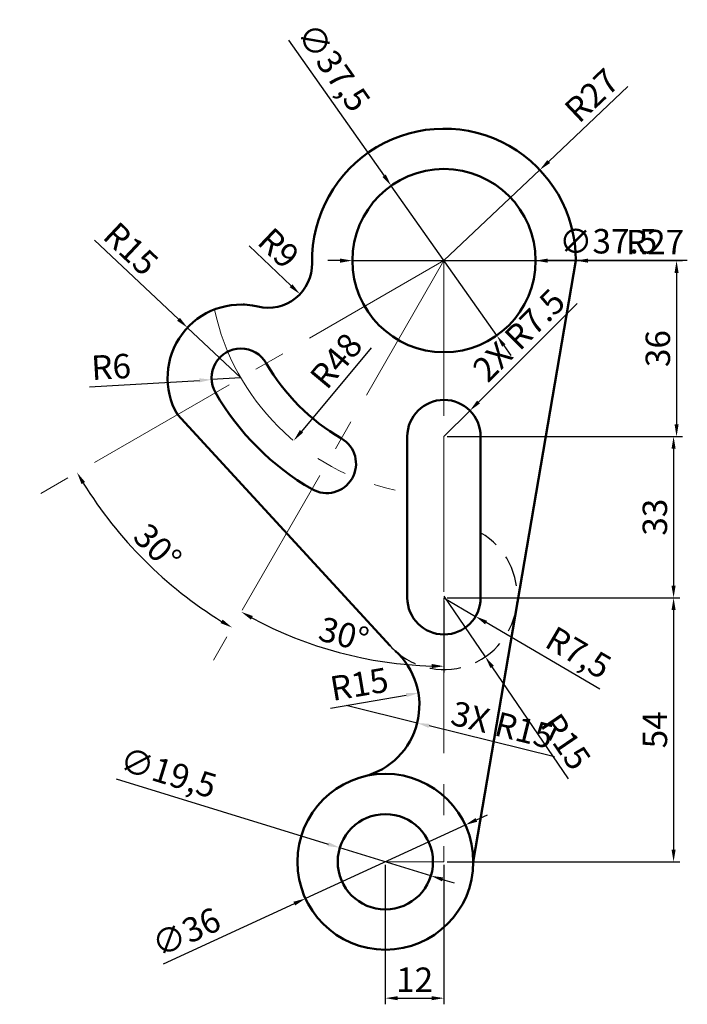
# Model space of a CAD drawing. Units: millimetres. Extents: x 3429 to 3566, y 1554 to 1755.
import ezdxf

# ---------------------------------------------------------------- set-up
doc = ezdxf.new("R2010")
doc.units = ezdxf.units.MM
doc.linetypes.add('CENTER', pattern=[50.8, 31.75, -6.35, 6.35, -6.35])
doc.linetypes.add('HIDDEN', pattern=[9.525, 6.35, -3.175])
for name, color, linetype, lineweight in [('M-CNTR', 4, 'CENTER', 18), ('M-DIMS', 2, 'Continuous', 25), ('M-HIDN', 7, 'HIDDEN', 25), ('M-OUTL', 7, 'Continuous', 50)]:
    doc.layers.add(name, color=color, linetype=linetype, lineweight=lineweight)
doc.styles.get("Standard").update_dxf_attribs({"font": 'arial.ttf'})
doc.dimstyles.new('ISO-25', dxfattribs={"dimtxt": 5, "dimasz": 2.5, "dimexe": 1.25, "dimexo": 0.625, "dimtad": 1, "dimtxsty": 'Standard', "dimcen": 2.5, "dimadec": 0, "dimazin": 0, "dimtfac": 1, "dimtmove": 0, "dimatfit": 3, "dimfxl": 1, "dimarcsym": 0})

# ---------------------------------------------------------------- blocks, each defined once
blk = doc.blocks.new('*D1')
at = {"layer": 'Defpoints', "color": 0, "transparency": 16777216}
for p in [(3516.16, 1705.91), (3516.16, 1669.91), (3563.76, 1669.91)]:
    blk.add_point(p, dxfattribs=at)
at = {"layer": 'M-DIMS', "color": 0, "lineweight": -2, "transparency": 16777216}
for p, q in [((3516.79, 1705.91), (3565.01, 1705.91)), ((3563.76, 1703.41), (3563.76, 1672.41)), ((3516.79, 1669.91), (3565.01, 1669.91))]:
    blk.add_line(p, q, dxfattribs=at)
at = {"layer": 'M-DIMS', "color": 0, "transparency": 16777216}
for points in [[(3563.35, 1703.41), (3564.18, 1703.41), (3563.76, 1705.91)], [(3563.35, 1672.41), (3564.18, 1672.41), (3563.76, 1669.91)]]:
    blk.add_solid(points, dxfattribs=at)
at = {"layer": 'M-DIMS', "color": 0, "transparency": 16777216, "insert": (3560.58, 1687.91), "char_height": 5, "attachment_point": 5, "rotation": 90}
blk.add_mtext('36', dxfattribs=at)
blk = doc.blocks.new('*D2')
at = {"layer": 'Defpoints', "color": 0, "transparency": 16777216}
for p in [(3516.16, 1669.91), (3516.16, 1636.91), (3563.15, 1636.91)]:
    blk.add_point(p, dxfattribs=at)
at = {"layer": 'M-DIMS', "color": 0, "lineweight": -2, "transparency": 16777216}
for p, q in [((3516.79, 1669.91), (3564.4, 1669.91)), ((3563.15, 1667.41), (3563.15, 1639.41)), ((3516.79, 1636.91), (3564.4, 1636.91))]:
    blk.add_line(p, q, dxfattribs=at)
at = {"layer": 'M-DIMS', "color": 0, "transparency": 16777216}
for points in [[(3562.73, 1667.41), (3563.57, 1667.41), (3563.15, 1669.91)], [(3562.73, 1639.41), (3563.57, 1639.41), (3563.15, 1636.91)]]:
    blk.add_solid(points, dxfattribs=at)
at = {"layer": 'M-DIMS', "color": 0, "transparency": 16777216, "insert": (3559.97, 1653.41), "char_height": 5, "attachment_point": 5, "rotation": 90}
blk.add_mtext('33', dxfattribs=at)
blk = doc.blocks.new('*D3')
at = {"layer": 'Defpoints', "color": 0, "transparency": 16777216}
for p in [(3516.16, 1636.91), (3516.16, 1582.91), (3563.15, 1582.91)]:
    blk.add_point(p, dxfattribs=at)
at = {"layer": 'M-DIMS', "color": 0, "lineweight": -2, "transparency": 16777216}
for p, q in [((3516.79, 1636.91), (3564.4, 1636.91)), ((3563.15, 1634.41), (3563.15, 1585.41)), ((3516.79, 1582.91), (3564.4, 1582.91))]:
    blk.add_line(p, q, dxfattribs=at)
at = {"layer": 'M-DIMS', "color": 0, "transparency": 16777216}
for points in [[(3562.73, 1634.41), (3563.57, 1634.41), (3563.15, 1636.91)], [(3562.73, 1585.41), (3563.57, 1585.41), (3563.15, 1582.91)]]:
    blk.add_solid(points, dxfattribs=at)
at = {"layer": 'M-DIMS', "color": 0, "transparency": 16777216, "insert": (3559.98, 1609.91), "char_height": 5, "attachment_point": 5, "rotation": 90}
blk.add_mtext('54', dxfattribs=at)
blk = doc.blocks.new('*D4')
at = {"layer": 'Defpoints', "color": 0, "transparency": 16777216}
for p in [(3504.16, 1582.91), (3516.16, 1582.91), (3516.16, 1555)]:
    blk.add_point(p, dxfattribs=at)
at = {"layer": 'M-DIMS', "color": 0, "lineweight": -2, "transparency": 16777216}
for p, q in [((3504.16, 1582.29), (3504.16, 1553.75)), ((3516.16, 1582.29), (3516.16, 1553.75)), ((3506.66, 1555), (3513.66, 1555))]:
    blk.add_line(p, q, dxfattribs=at)
at = {"layer": 'M-DIMS', "color": 0, "transparency": 16777216}
for points in [[(3506.66, 1555.41), (3506.66, 1554.58), (3504.16, 1555)], [(3513.66, 1555.41), (3513.66, 1554.58), (3516.16, 1555)]]:
    blk.add_solid(points, dxfattribs=at)
at = {"layer": 'M-DIMS', "color": 0, "transparency": 16777216, "insert": (3510.16, 1558.13), "char_height": 5, "attachment_point": 5}
blk.add_mtext('12', dxfattribs=at)
blk = doc.blocks.new('*D5')
at = {"layer": 'Defpoints', "color": 0, "transparency": 16777216}
for p in [(3516.16, 1705.91), (3516.16, 1669.91), (3516.16, 1636.91), (3487.78, 1627.93), (3468.96, 1624.15)]:
    blk.add_point(p, dxfattribs=at)
at = {"layer": 'M-DIMS', "color": 0, "lineweight": -2, "transparency": 16777216}
blk.add_line((3516.16, 1636.29), (3516.16, 1621.67), dxfattribs=at)
blk.add_arc((3516.16, 1705.91), 82.99, 241.7261, 268.2739, dxfattribs=at)
at = {"layer": 'M-DIMS', "color": 0, "transparency": 16777216}
for points in [[(3476.65, 1632.46), (3477.06, 1633.19), (3474.67, 1634.04)], [(3513.67, 1623.38), (3513.66, 1622.54), (3516.16, 1622.92)]]:
    blk.add_solid(points, dxfattribs=at)
at = {"layer": 'M-DIMS', "color": 0, "transparency": 16777216, "insert": (3495.51, 1628.82), "char_height": 5, "attachment_point": 5, "rotation": 345}
blk.add_mtext('30°', dxfattribs=at)
blk = doc.blocks.new('*D6')
at = {"layer": 'Defpoints', "color": 0, "transparency": 16777216}
for p in [(3535.78, 1724.47), (3516.16, 1705.91)]:
    blk.add_point(p, dxfattribs=at)
at = {"layer": 'M-DIMS', "color": 0, "lineweight": -2, "transparency": 16777216}
for p, q in [((3553.79, 1741.51), (3537.59, 1726.18)), ((3516.16, 1705.91), (3535.78, 1724.47))]:
    blk.add_line(p, q, dxfattribs=at)
at = {"layer": 'M-DIMS', "color": 0, "transparency": 16777216}
blk.add_solid([(3537.31, 1726.49), (3537.88, 1725.88), (3535.78, 1724.47)], dxfattribs=at)
at = {"layer": 'M-DIMS', "color": 0, "transparency": 16777216, "insert": (3546.85, 1739.25), "char_height": 5, "attachment_point": 5, "rotation": 43.4094}
blk.add_mtext('R27', dxfattribs=at)
blk = doc.blocks.new('*D7')
at = {"layer": 'Defpoints', "color": 0, "transparency": 16777216}
for p in [(3510.92, 1617.43), (3496.13, 1614.92)]:
    blk.add_point(p, dxfattribs=at)
at = {"layer": 'M-DIMS', "color": 0, "lineweight": -2, "transparency": 16777216}
blk.add_line((3492.94, 1614.37), (3508.45, 1617.01), dxfattribs=at)
at = {"layer": 'M-DIMS', "color": 0, "transparency": 16777216}
blk.add_solid([(3508.38, 1617.42), (3508.52, 1616.6), (3510.92, 1617.43)], dxfattribs=at)
at = {"layer": 'M-DIMS', "color": 0, "transparency": 16777216, "insert": (3498.93, 1618.62), "char_height": 5, "attachment_point": 5, "rotation": 9.6568}
blk.add_mtext('R15', dxfattribs=at)
blk = doc.blocks.new('*D8')
at = {"layer": 'Defpoints', "color": 0, "transparency": 16777216}
for p in [(3516.16, 1636.91), (3522.63, 1633.12)]:
    blk.add_point(p, dxfattribs=at)
at = {"layer": 'M-DIMS', "color": 0, "lineweight": -2, "transparency": 16777216}
for p, q in [((3516.16, 1636.91), (3522.63, 1633.12)), ((3548.08, 1618.2), (3524.79, 1631.85))]:
    blk.add_line(p, q, dxfattribs=at)
at = {"layer": 'M-DIMS', "color": 0, "transparency": 16777216}
blk.add_solid([(3525, 1632.21), (3524.58, 1631.49), (3522.63, 1633.12)], dxfattribs=at)
at = {"layer": 'M-DIMS', "color": 0, "transparency": 16777216, "insert": (3543.37, 1625.16), "char_height": 5, "attachment_point": 5, "rotation": 329.6153}
blk.add_mtext('R7,5', dxfattribs=at)
blk = doc.blocks.new('*D9')
at = {"layer": 'Defpoints', "color": 0, "transparency": 16777216}
for p in [(3516.16, 1637.25), (3524.61, 1624.85)]:
    blk.add_point(p, dxfattribs=at)
at = {"layer": 'M-DIMS', "color": 0, "lineweight": -2, "transparency": 16777216}
for p, q in [((3516.16, 1637.25), (3524.61, 1624.85)), ((3541.66, 1599.85), (3526.02, 1622.79))]:
    blk.add_line(p, q, dxfattribs=at)
at = {"layer": 'M-DIMS', "color": 0, "transparency": 16777216}
blk.add_solid([(3526.37, 1623.02), (3525.68, 1622.55), (3524.61, 1624.85)], dxfattribs=at)
at = {"layer": 'M-DIMS', "color": 0, "transparency": 16777216, "insert": (3540.56, 1607.11), "char_height": 5, "attachment_point": 5, "rotation": 304.2901}
blk.add_mtext('R15', dxfattribs=at)
blk = doc.blocks.new('*D10')
at = {"layer": 'Defpoints', "color": 0, "transparency": 16777216}
for p in [(3516.16, 1705.91), (3485.4, 1669.06)]:
    blk.add_point(p, dxfattribs=at)
at = {"layer": 'M-DIMS', "color": 0, "lineweight": -2, "transparency": 16777216}
blk.add_line((3501.25, 1688.04), (3487, 1670.98), dxfattribs=at)
at = {"layer": 'M-DIMS', "color": 0, "transparency": 16777216}
blk.add_solid([(3486.68, 1671.25), (3487.32, 1670.72), (3485.4, 1669.06)], dxfattribs=at)
at = {"layer": 'M-DIMS', "color": 0, "transparency": 16777216, "insert": (3494.58, 1685.01), "char_height": 5, "attachment_point": 5, "rotation": 50.1415}
blk.add_mtext('R48', dxfattribs=at)
blk = doc.blocks.new('*D11')
at = {"layer": 'Defpoints', "color": 0, "transparency": 16777216}
for p in [(3468.6, 1681.56), (3474.59, 1681.91)]:
    blk.add_point(p, dxfattribs=at)
at = {"layer": 'M-DIMS', "color": 0, "lineweight": -2, "transparency": 16777216}
for p, q in [((3443.61, 1680.1), (3466.11, 1681.41)), ((3474.59, 1681.91), (3468.6, 1681.56))]:
    blk.add_line(p, q, dxfattribs=at)
at = {"layer": 'M-DIMS', "color": 0, "transparency": 16777216}
blk.add_solid([(3466.08, 1681.83), (3466.13, 1681), (3468.6, 1681.56)], dxfattribs=at)
at = {"layer": 'M-DIMS', "color": 0, "transparency": 16777216, "insert": (3448.07, 1683.54), "char_height": 5, "attachment_point": 5, "rotation": 3.3514}
blk.add_mtext('R6', dxfattribs=at)
blk = doc.blocks.new('*D12')
at = {"layer": 'Defpoints', "color": 0, "transparency": 16777216}
for p in [(3463.67, 1692.19), (3474.59, 1681.91)]:
    blk.add_point(p, dxfattribs=at)
at = {"layer": 'M-DIMS', "color": 0, "lineweight": -2, "transparency": 16777216}
for p, q in [((3444.65, 1710.08), (3461.85, 1693.9)), ((3474.59, 1681.91), (3463.67, 1692.19))]:
    blk.add_line(p, q, dxfattribs=at)
at = {"layer": 'M-DIMS', "color": 0, "transparency": 16777216}
blk.add_solid([(3462.13, 1694.2), (3461.56, 1693.6), (3463.67, 1692.19)], dxfattribs=at)
at = {"layer": 'M-DIMS', "color": 0, "transparency": 16777216, "insert": (3451.65, 1707.86), "char_height": 5, "attachment_point": 5, "rotation": 316.7505}
blk.add_mtext('R15', dxfattribs=at)
blk = doc.blocks.new('*D13')
at = {"layer": 'Defpoints', "color": 0, "transparency": 16777216}
for p in [(3480.17, 1705.25), (3486.69, 1699.05)]:
    blk.add_point(p, dxfattribs=at)
at = {"layer": 'M-DIMS', "color": 0, "lineweight": -2, "transparency": 16777216}
blk.add_line((3476.31, 1708.92), (3484.88, 1700.77), dxfattribs=at)
at = {"layer": 'M-DIMS', "color": 0, "transparency": 16777216}
blk.add_solid([(3485.16, 1701.07), (3484.59, 1700.47), (3486.69, 1699.05)], dxfattribs=at)
at = {"layer": 'M-DIMS', "color": 0, "transparency": 16777216, "insert": (3481.88, 1708.01), "char_height": 5, "attachment_point": 5, "rotation": 316.4015}
blk.add_mtext('R9', dxfattribs=at)
blk = doc.blocks.new('*D14')
at = {"layer": 'Defpoints', "color": 0, "transparency": 16777216}
for p in [(3505.36, 1721.23), (3526.97, 1690.59)]:
    blk.add_point(p, dxfattribs=at)
at = {"layer": 'M-DIMS', "color": 0, "lineweight": -2, "transparency": 16777216}
for p, q in [((3484.34, 1751.03), (3503.92, 1723.28)), ((3526.97, 1690.59), (3505.36, 1721.23)), ((3528.41, 1688.54), (3529.85, 1686.5))]:
    blk.add_line(p, q, dxfattribs=at)
at = {"layer": 'M-DIMS', "color": 0, "transparency": 16777216}
for points in [[(3504.26, 1723.52), (3503.58, 1723.04), (3505.36, 1721.23)], [(3528.75, 1688.79), (3528.07, 1688.3), (3526.97, 1690.59)]]:
    blk.add_solid(points, dxfattribs=at)
at = {"layer": 'M-DIMS', "color": 0, "transparency": 16777216, "insert": (3493.06, 1745.11), "char_height": 5, "attachment_point": 5, "rotation": 305.194}
blk.add_mtext('∅37,5', dxfattribs=at)
blk = doc.blocks.new('*D15')
at = {"layer": 'Defpoints', "color": 0, "transparency": 16777216}
for p in [(3494.85, 1585.78), (3513.48, 1580.04)]:
    blk.add_point(p, dxfattribs=at)
at = {"layer": 'M-DIMS', "color": 0, "lineweight": -2, "transparency": 16777216}
for p, q in [((3449.05, 1599.89), (3492.46, 1586.52)), ((3513.48, 1580.04), (3494.85, 1585.78)), ((3515.87, 1579.3), (3518.26, 1578.57))]:
    blk.add_line(p, q, dxfattribs=at)
at = {"layer": 'M-DIMS', "color": 0, "transparency": 16777216}
for points in [[(3492.58, 1586.92), (3492.33, 1586.12), (3494.85, 1585.78)], [(3515.99, 1579.7), (3515.75, 1578.91), (3513.48, 1580.04)]]:
    blk.add_solid(points, dxfattribs=at)
at = {"layer": 'M-DIMS', "color": 0, "transparency": 16777216, "insert": (3459.57, 1600.53), "char_height": 5, "attachment_point": 5, "rotation": 342.8759}
blk.add_mtext('∅19,5', dxfattribs=at)
blk = doc.blocks.new('*D16')
at = {"layer": 'Defpoints', "color": 0, "transparency": 16777216}
for p in [(3520.52, 1590.43), (3487.81, 1575.39)]:
    blk.add_point(p, dxfattribs=at)
at = {"layer": 'M-DIMS', "color": 0, "lineweight": -2, "transparency": 16777216}
for p, q in [((3522.79, 1591.47), (3525.06, 1592.52)), ((3520.52, 1590.43), (3487.81, 1575.39)), ((3458.76, 1562.03), (3485.54, 1574.35))]:
    blk.add_line(p, q, dxfattribs=at)
at = {"layer": 'M-DIMS', "color": 0, "transparency": 16777216}
for points in [[(3522.62, 1591.85), (3522.96, 1591.1), (3520.52, 1590.43)], [(3485.36, 1574.73), (3485.71, 1573.97), (3487.81, 1575.39)]]:
    blk.add_solid(points, dxfattribs=at)
at = {"layer": 'M-DIMS', "color": 0, "transparency": 16777216, "insert": (3463.66, 1567.94), "char_height": 5, "attachment_point": 5, "rotation": 24.6931}
blk.add_mtext('∅36', dxfattribs=at)
blk = doc.blocks.new('*D17')
at = {"layer": 'Defpoints', "color": 0, "transparency": 16777216}
for p in [(3516.16, 1705.91), (3516.16, 1705.91), (3429.33, 1655.78), (3449.74, 1650.17), (3468.96, 1624.15)]:
    blk.add_point(p, dxfattribs=at)
at = {"layer": 'M-DIMS', "color": 0, "lineweight": -2, "transparency": 16777216}
blk.add_arc((3516.16, 1705.91), 86.71, 211.652, 238.348, dxfattribs=at)
at = {"layer": 'M-DIMS', "color": 0, "transparency": 16777216}
for points in [[(3441.99, 1660.19), (3442.71, 1660.62), (3441.07, 1662.55)], [(3470.87, 1632.46), (3470.45, 1631.74), (3472.81, 1630.82)]]:
    blk.add_solid(points, dxfattribs=at)
at = {"layer": 'M-DIMS', "color": 0, "transparency": 16777216, "insert": (3457.1, 1646.84), "char_height": 5, "attachment_point": 5, "rotation": 315}
blk.add_mtext('30°', dxfattribs=at)
blk = doc.blocks.new('*D18')
at = {"layer": 'Defpoints', "color": 0, "transparency": 16777216}
for p in [(3497.41, 1705.91), (3534.91, 1705.91)]:
    blk.add_point(p, dxfattribs=at)
at = {"layer": 'M-DIMS', "color": 0, "lineweight": -2, "transparency": 16777216}
for p, q in [((3494.91, 1705.91), (3492.41, 1705.91)), ((3497.41, 1705.91), (3534.91, 1705.91)), ((3559.63, 1705.91), (3537.41, 1705.91))]:
    blk.add_line(p, q, dxfattribs=at)
at = {"layer": 'M-DIMS', "color": 0, "transparency": 16777216}
for points in [[(3494.91, 1706.33), (3494.91, 1705.49), (3497.41, 1705.91)], [(3537.41, 1706.33), (3537.41, 1705.49), (3534.91, 1705.91)]]:
    blk.add_solid(points, dxfattribs=at)
at = {"layer": 'M-DIMS', "color": 0, "transparency": 16777216, "insert": (3549.77, 1709.23), "char_height": 5, "attachment_point": 5, "rotation": 0.0014}
blk.add_mtext('∅37.5', dxfattribs=at)
blk = doc.blocks.new('*D19')
at = {"layer": 'Defpoints', "color": 0, "transparency": 16777216}
for p in [(3516.16, 1705.91), (3543.16, 1705.91)]:
    blk.add_point(p, dxfattribs=at)
at = {"layer": 'M-DIMS', "color": 0, "lineweight": -2, "transparency": 16777216}
for p, q in [((3516.16, 1705.91), (3543.16, 1705.91)), ((3565.96, 1705.91), (3545.66, 1705.91))]:
    blk.add_line(p, q, dxfattribs=at)
at = {"layer": 'M-DIMS', "color": 0, "transparency": 16777216}
blk.add_solid([(3545.66, 1706.33), (3545.66, 1705.49), (3543.16, 1705.91)], dxfattribs=at)
at = {"layer": 'M-DIMS', "color": 0, "transparency": 16777216, "insert": (3559.36, 1709.05), "char_height": 5, "attachment_point": 5, "rotation": 0.001}
blk.add_mtext('R27', dxfattribs=at)
blk = doc.blocks.new('*D20')
at = {"layer": 'Defpoints', "color": 0, "transparency": 16777216}
for p in [(3496.13, 1614.92), (3510.69, 1611.31)]:
    blk.add_point(p, dxfattribs=at)
at = {"layer": 'M-DIMS', "color": 0, "lineweight": -2, "transparency": 16777216}
for p, q in [((3496.13, 1614.92), (3510.69, 1611.31)), ((3538.81, 1604.35), (3513.11, 1610.71))]:
    blk.add_line(p, q, dxfattribs=at)
at = {"layer": 'M-DIMS', "color": 0, "transparency": 16777216}
blk.add_solid([(3513.22, 1611.12), (3513.01, 1610.31), (3510.69, 1611.31)], dxfattribs=at)
at = {"layer": 'M-DIMS', "color": 0, "transparency": 16777216, "insert": (3527.94, 1610.32), "char_height": 5, "attachment_point": 5, "rotation": 346.0971}
blk.add_mtext('3X R15', dxfattribs=at)
blk = doc.blocks.new('*D21')
at = {"layer": 'Defpoints', "color": 0, "transparency": 16777216}
for p in [(3521.47, 1675.21), (3516.16, 1669.91)]:
    blk.add_point(p, dxfattribs=at)
at = {"layer": 'M-DIMS', "color": 0, "lineweight": -2, "transparency": 16777216}
for p, q in [((3543.39, 1697.14), (3523.23, 1676.98)), ((3516.16, 1669.91), (3521.47, 1675.21))]:
    blk.add_line(p, q, dxfattribs=at)
at = {"layer": 'M-DIMS', "color": 0, "transparency": 16777216}
blk.add_solid([(3522.94, 1677.28), (3523.53, 1676.69), (3521.47, 1675.21)], dxfattribs=at)
at = {"layer": 'M-DIMS', "color": 0, "transparency": 16777216, "insert": (3531.95, 1690.19), "char_height": 5, "attachment_point": 5, "rotation": 45.0014}
blk.add_mtext('2X R7.5', dxfattribs=at)

msp = doc.modelspace()

# ---------------------------------------------------------------- linework, layer by layer
at = {"layer": 'M-CNTR'}
for p, q in [((3516.164, 1705.911), (3429.332, 1655.778)), ((3516.164, 1705.911), (3468.962, 1624.154)), ((3516.164, 1705.911), (3516.164, 1669.911)), ((3516.164, 1669.911), (3516.164, 1636.911)), ((3516.164, 1636.911), (3516.164, 1582.911)), ((3516.164, 1582.911), (3504.164, 1582.911))]:
    msp.add_line(p, q, dxfattribs=at)
msp.add_arc((3516.164, 1705.911), 48, 192.0214, 257.9786, dxfattribs=at)
at = {"layer": 'M-HIDN'}
msp.add_arc((3516.164, 1637.245), 15, 222.60443, 60, dxfattribs=at)
at = {"layer": 'M-OUTL'}
for p, q in [((3543.164, 1705.911), (3522.164, 1582.911)), ((3461.604, 1674.411), (3505.123, 1627.091)), ((3508.664, 1669.911), (3508.664, 1636.911)), ((3523.664, 1669.911), (3523.664, 1636.911))]:
    msp.add_line(p, q, dxfattribs=at)
for centre, radius in [((3516.164, 1705.911), 18.75), ((3504.164, 1582.911), 18), ((3504.164, 1582.911), 9.75)]:
    msp.add_circle(centre, radius, dxfattribs=at)
for centre, radius, start, end in [((3516.164, 1705.911), 27, 0, 181.04498), ((3480.17, 1705.254), 9, 256.56746, 1.04498), ((3474.595, 1681.911), 15, 76.56746, 210), ((3516.164, 1705.911), 42, 192.0214, 192.38756), ((3474.595, 1681.911), 6, 30, 210), ((3516.164, 1705.911), 42, 210, 240), ((3516.164, 1705.911), 54, 210, 240), ((3516.164, 1669.911), 7.5, 0, 180), ((3492.164, 1664.341), 6, 240, 60), ((3516.164, 1636.911), 7.5, 180, 0), ((3496.128, 1614.917), 15, 284.09439, 48.09697)]:
    msp.add_arc(centre, radius, start, end, dxfattribs=at)

# ---------------------------------------------------------------- dimensions: what is measured, and where the dimension line sits
at = {"layer": 'M-DIMS'}
for p1, p2, override, picture, middle in [((3526.97, 1690.588), (3505.357, 1721.233), {"dimclrd": 0, "dimclre": 0, "dimclrt": 0}, '*D14', (3490.024, 1742.974)), ((3497.414, 1705.91), (3534.914, 1705.911), {"dimdec": 1, "dimlfac": 1, "dimrnd": 0, "dimzin": 0, "dimdsep": 46, "dimlunit": 2}, '*D18', (3549.771, 1705.911)), ((3513.482, 1580.04), (3494.846, 1585.781), {"dimclrd": 0, "dimclre": 0, "dimclrt": 0}, '*D15', (3458.474, 1596.988)), ((3520.518, 1590.43), (3487.81, 1575.391), {"dimclrd": 0, "dimclre": 0, "dimclrt": 0}, '*D16', (3465.049, 1564.926))]:
    dim = msp.add_diameter_dim_2p(p1=p1, p2=p2, dimstyle='ISO-25', override=override, dxfattribs=at)
    dim.commit()
    dim.dimension.update_dxf_attribs({"geometry": picture, "text_midpoint": middle, "dimtype": 163})
for center, mpoint, override, picture, middle in [((3516.164, 1705.911), (3535.778, 1724.465), {"dimclrd": 0, "dimclre": 0, "dimclrt": 0}, '*D6', (3549.001, 1736.973)), ((3474.595, 1681.911), (3463.669, 1692.188), {"dimclrd": 0, "dimclre": 0, "dimclrt": 0}, '*D12', (3449.47, 1705.545)), ((3480.17, 1705.254), (3486.687, 1699.048), {"dimclrd": 0, "dimclre": 0, "dimclrt": 0}, '*D13', (3479.691, 1705.71)), ((3516.164, 1705.911), (3543.164, 1705.911), {"dimdec": 0, "dimlfac": 1, "dimrnd": 0, "dimzin": 0, "dimdsep": 46, "dimlunit": 2}, '*D19', (3559.364, 1705.911)), ((3516.164, 1705.911), (3485.401, 1669.064), {"dimclrd": 0, "dimclre": 0, "dimclrt": 0}, '*D10', (3497.014, 1682.974)), ((3474.595, 1681.911), (3468.605, 1681.56), {"dimclrd": 0, "dimclre": 0, "dimclrt": 0}, '*D11', (3448.256, 1680.368)), ((3516.164, 1637.245), (3524.615, 1624.852), {"dimclrd": 0, "dimclre": 0, "dimclrt": 0}, '*D9', (3537.934, 1605.319)), ((3516.164, 1636.911), (3522.634, 1633.117), {"dimclrd": 0, "dimclre": 0, "dimclrt": 0}, '*D8', (3541.537, 1622.033)), ((3496.128, 1614.917), (3510.915, 1617.433), {"dimclrd": 0, "dimclre": 0, "dimclrt": 0}, '*D7', (3499.462, 1615.484))]:
    dim = msp.add_radius_dim(center=center, mpoint=mpoint, dimstyle='ISO-25', override=override, dxfattribs=at)
    dim.commit()
    dim.dimension.update_dxf_attribs({"geometry": picture, "text_midpoint": middle, "dimtype": 164})
for base, line1, line2, picture, middle in [((3449.739, 1650.174), ((3516.164, 1705.911), (3468.962, 1624.154)), ((3516.164, 1705.911), (3429.332, 1655.778)), '*D17', (3457.098, 1646.845)), ((3487.78, 1627.926), ((3516.164, 1669.911), (3516.164, 1636.911)), ((3516.164, 1705.911), (3468.962, 1624.154)), '*D5', (3495.508, 1628.82))]:
    dim = msp.add_angular_dim_2l(base=base, line1=line1, line2=line2, dimstyle='ISO-25', override={"dimclrd": 0, "dimclre": 0, "dimclrt": 0}, dxfattribs=at)
    dim.commit()
    dim.dimension.update_dxf_attribs({"geometry": picture, "text_midpoint": middle})
for base, p1, p2, picture, middle in [((3563.763, 1669.911), (3516.164, 1705.911), (3516.164, 1669.911), '*D1', (3560.584, 1687.911)), ((3563.149, 1636.911), (3516.164, 1669.911), (3516.164, 1636.911), '*D2', (3559.97, 1653.411)), ((3563.149, 1582.911), (3516.164, 1636.911), (3516.164, 1582.911), '*D3', (3559.982, 1609.911))]:
    dim = msp.add_linear_dim(base=base, p1=p1, p2=p2, angle=90, dimstyle='ISO-25', override={"dimclrd": 0, "dimclre": 0, "dimclrt": 0}, dxfattribs=at)
    dim.commit()
    dim.dimension.update_dxf_attribs({"geometry": picture, "text_midpoint": middle})
for center, mpoint, text, override, picture, middle in [((3516.164, 1669.911), (3521.467, 1675.214), '2X <>', {"dimdec": 1, "dimlfac": 1, "dimrnd": 0, "dimzin": 0, "dimdsep": 46, "dimlunit": 2}, '*D21', (3531.949, 1690.191)), ((3496.128, 1614.917), (3510.688, 1611.313), '3X <>', {"dimdec": 0, "dimlfac": 1, "dimrnd": 0, "dimzin": 0, "dimdsep": 46, "dimlunit": 2}, '*D20', (3527.942, 1610.318))]:
    dim = msp.add_radius_dim(center=center, mpoint=mpoint, text=text, dimstyle='ISO-25', override=override, dxfattribs=at)
    dim.commit()
    dim.dimension.update_dxf_attribs({"geometry": picture, "text_midpoint": middle})
dim = msp.add_linear_dim(base=(3516.164, 1554.995), p1=(3504.164, 1582.911), p2=(3516.164, 1582.911), dimstyle='ISO-25', override={"dimclrd": 0, "dimclre": 0, "dimclrt": 0}, dxfattribs=at)
dim.commit()
dim.dimension.update_dxf_attribs({"geometry": '*D4', "text_midpoint": (3510.164, 1558.13)})

doc.saveas('drawing.dxf')
